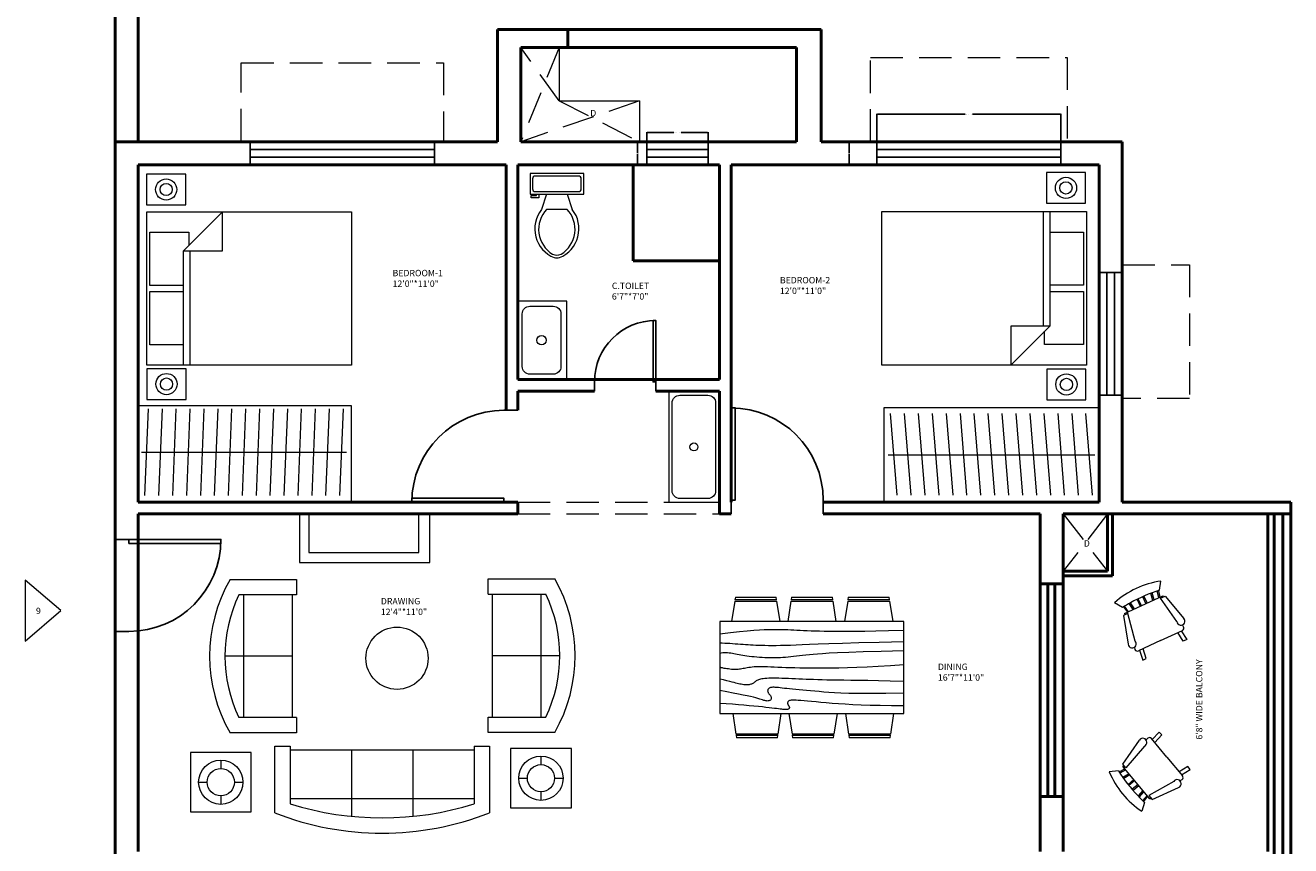
# Model space of a CAD drawing. Units: inches. Extents: x 4795 to 6024, y 2716 to 5025.
# Tile 16 of 19: x 5493 to 5988, y 4094 to 4414. Entities that reach past the tile are written whole.
import ezdxf

# ---------------------------------------------------------------- set-up
doc = ezdxf.new("R2010")
doc.units = ezdxf.units.IN
doc.linetypes.add('DASHED', pattern=[19.05, 12.7, -6.35])
for name, color, linetype, lineweight in [('A-ANNO-DIMS', 2, 'Continuous', 18), ('A-ANNO-TEXT', 7, 'Continuous', 18), ('A-AREA-IDEN', 3, 'Continuous', 18), ('A-DOOR', 4, 'Continuous', 25), ('A-FLOR-FIXT', 9, 'Continuous', 18), ('A-FURN', 8, 'Continuous', 18), ('A-GLAZ', 4, 'Continuous', 25), ('A-WALL', 7, 'Continuous', 50), ('A-WALL-OVHD', 8, 'DASHED', 18)]:
    doc.layers.add(name, color=color, linetype=linetype, lineweight=lineweight)
doc.styles.get("Standard").update_dxf_attribs({"font": 'arial.ttf'})
doc.dimstyles.get("Standard").update_dxf_attribs({"dimtxt": 0.18, "dimasz": 0.18, "dimexe": 0.18, "dimexo": 0.0625, "dimgap": 0.09, "dimtad": 0, "dimtih": 1, "dimtoh": 1, "dimdec": 4, "dimzin": 0, "dimdsep": 46, "dimtxsty": 'Standard', "dimcen": 0.09, "dimadec": 0, "dimazin": 0, "dimtfac": 1, "dimtdec": 4, "dimtofl": 0, "dimtmove": 0, "dimatfit": 3, "dimfxl": 1, "dimtolj": 1, "dimtzin": 0, "dimarcsym": 0})

# ---------------------------------------------------------------- blocks, each defined once
blk = doc.blocks.new('*U2')
for p, q in [((0, 0), (0, -6)), ((40, 0), (40, -6))]:
    blk.add_line(p, q)
blk.add_lwpolyline([(0, 0), (0, 40), (1.75, 40), (1.75, 0)], close=True)
blk.add_arc((0, 0), 40, 0, 90)
blk = doc.blocks.new('Bed - Queen')
for p, q in [((0, -80.00003), (0, 0)), ((0, 0), (59.99999, 0)), ((59.99999, 0), (59.99999, -80.00003)), ((7.99999, -1.2), (28.79998, -1.2)), ((7.99999, -14.4), (7.99999, -1.2)), ((28.79998, -1.2), (28.79998, -14.4)), ((31.19999, -1.2), (51.99999, -1.2)), ((31.19999, -14.4), (31.19999, -1.2)), ((51.99999, -1.2), (51.99999, -16.4)), ((0, -14.4), (44.8, -14.4)), ((59.99999, -29.6), (44.8, -14.4)), ((44.8, -14.4), (44.8, -29.6)), ((44.8, -16.8), (0, -16.8)), ((51.99999, -16.4), (46.79936, -16.4)), ((44.8, -29.6), (59.99999, -29.6)), ((59.99999, -80.00003), (0, -80.00003))]:
    blk.add_line(p, q)
blk = doc.blocks.new('Toilet - top')
for p, q in [((9.5, -6), (9.5, -2)), ((-10, -8.5), (-8, -8.5)), ((-10, -9.5), (-10, -8.5)), ((-7, -9.5), (-10, -9.5)), ((-8, -8.5), (-8, -8)), ((-7, -8), (-7, -9.5)), ((-4, -8), (-6, -14)), ((4, -8), (6, -14)), ((4, -14), (-4, -14))]:
    blk.add_line(p, q)
blk.add_lwpolyline([(10.5, -8), (10.5, 0), (-10.5, 0), (-10.5, -8)], close=True)
for points in [[(-9.5, -2), (-9.5, -6)], [(8.5, -1), (-8.5, -1)], [(-8.5, -7), (8.5, -7)]]:
    blk.add_lwpolyline(points)
for centre, radius, start, end in [((-8.62, -1.88), 0.884, 81.8699, 188.1301), ((8.62, -1.88), 0.884, 351.8699, 98.1301), ((-8.62, -6.12), 0.884, 171.8699, 278.1301), ((8.62, -6.12), 0.884, 261.8699, 8.1301), ((3.52, -21.58), 12.17, 141.4691, 247.9714), ((4.2, -21.82), 11.33, 136.3677, 238.9468), ((-3.52, -21.58), 12.17, 292.0284, 38.5307), ((-4.2, -21.82), 11.33, 301.053, 43.6321), ((0, -27.88), 4, 245.7318, 294.2682), ((0, -29), 4, 254.8605, 285.1395)]:
    blk.add_arc(centre, radius, start, end)
blk = doc.blocks.new('Sofa - Roundback 7 ft.')
for p, q in [((-12.00002, -32.4421), (-12.00003, -6.5971)), ((11.99997, -32.4421), (11.99998, -6.5971)), ((-36.000027, -34), (-36.000027, -11.4696)), ((-35.999844, -13.3819), (35.9998, -13.3819)), ((35.99998, -34), (35.99998, -11.4696)), ((-36.000027, -32.4421), (35.99998, -32.4421))]:
    blk.add_line(p, q)
for points in [[(-36.000027, -34), (-42.000027, -34), (-42.000027, -8)], [(41.99998, -8), (41.99998, -34), (35.99998, -34)]]:
    blk.add_lwpolyline(points)
for centre, radius, start, end in [((0, -114.25), 114.25, 68.43141, 111.5686), ((-0.00001, -127.1968), 121.1968, 72.72033, 107.2797)]:
    blk.add_arc(centre, radius, start, end)
blk = doc.blocks.new('Sofa - Roundback Loveseat 5 ft.')
for p, q in [((0, -32.44198), (0, -5.99998)), ((-24, -33.99998), (-24, -11.46958)), ((-23.9998, -13.38178), (23.99986, -13.38178)), ((24.00004, -33.99998), (24.00004, -11.46958)), ((-24, -32.44198), (24.00004, -32.44198))]:
    blk.add_line(p, q)
for points in [[(-24, -33.99998), (-30, -33.99998), (-30, -7.99998)], [(30.00004, -7.99998), (30.00004, -33.99998), (24.00004, -33.99998)]]:
    blk.add_lwpolyline(points)
for centre, radius, start, end in [((0, -60.24998), 60.24998, 60.13715, 119.8628), ((0, -61.38438), 55.38444, 64.32083, 115.6792)]:
    blk.add_arc(centre, radius, start, end)
blk = doc.blocks.new('Chair - Rocking')
for p, q in [((-8, -4.5), (-10, -1.5)), ((-7.5, -4.5), (-7, -7)), ((-6.5, -7), (-7.02225, -4.43)), ((-4.5, -7), (-4.96674, -4.19951)), ((-4, -7), (-4.40532, -4.16272)), ((-1.5, -4.05012), (-1.5, -7)), ((-1, -7), (-1, -4.05012)), ((1, -7), (1, -4.04655)), ((1.5, -4.05012), (1.5, -7)), ((4, -7), (4.40187, -4.18694)), ((4.5, -7), (4.96761, -4.19437)), ((6.5, -7), (7, -4.4057)), ((7.5, -4.5), (7, -7)), ((8, -4.5), (10, -1.5)), ((-9, -7.5), (-12, -18.49999)), ((-7, -7.5), (-9, -7.5)), ((-9, -18.49999), (-7, -7.5)), ((-8.23428, -6.99939), (-8.3093, -7.47958)), ((-8.23041, -7), (8.23915, -7)), ((7, -7.5), (9, -7.5)), ((9, -18.49999), (7, -7.5)), ((8.31071, -7.48854), (8.23449, -7.00073)), ((9, -7.5), (12, -18.49999)), ((-10.36644, -20.64523), (-10.5, -21.49999)), ((-9, -22.49999), (-9.5, -26.49999)), ((0, -22.49999), (-9.5, -22.49999)), ((-8, -26.49999), (-7.5, -22.49999)), ((0, -22.49999), (9.5, -22.49999)), ((8, -26.49999), (7.5, -22.49999)), ((9, -22.49999), (9.5, -26.49999)), ((10.5, -21.49999), (10.3575, -20.58798)), ((-9.5, -26.49999), (-8, -26.49999)), ((9.5, -26.49999), (8, -26.49999))]:
    blk.add_line(p, q)
for centre, radius, start, end in [((0, -34.08333), 34.08333, 72.93847, 107.0615), ((0, -68.25004), 64.25, 93.92211, 97.15267), ((0, -68.25004), 64.25, 82.84733, 93.92211), ((-10.5, -18.99999), 1.58114, 161.5651, 18.43495), ((10.5, -18.99999), 1.58114, 161.5651, 18.43495), ((-9.5, -21.49999), 1, 180, 270), ((9.5, -21.49999), 1, 270, 0)]:
    blk.add_arc(centre, radius, start, end)
blk = doc.blocks.new('WIN-48')
for p, q in [((0, 0), (0, 48)), ((0, 48), (9, 48)), ((3, 0), (3, 48)), ((6, 48), (6, 0)), ((9, 48), (9, 0)), ((9, 0), (0, 0))]:
    blk.add_line(p, q)
blk = doc.blocks.new('WIN-72')
for p, q in [((0, 0), (0, 9)), ((0, 9), (72, 9)), ((0, 6), (72, 6)), ((72, 9), (72, 0)), ((72, 3), (0, 3)), ((72, 0), (0, 0))]:
    blk.add_line(p, q)
blk = doc.blocks.new('WIN-24')
for p, q in [((0, 0), (0, 9)), ((0, 9), (24, 9)), ((0, 6), (24, 6)), ((24, 9), (24, 0)), ((24, 3), (0, 3)), ((24, 0), (0, 0))]:
    blk.add_line(p, q)
blk = doc.blocks.new('CHAIR-DINING')
for p, q in [((8, 17.72), (0, 18.97)), ((8, 17.71), (8, 1.25)), ((9.5, 17.48), (8.5, 17.64)), ((8.5, 1.33), (8.5, 17.64)), ((9.5, 17.48), (9.5, 1.48)), ((0, 0), (8, 1.25)), ((8.5, 1.33), (9.5, 1.48))]:
    blk.add_line(p, q)
blk = doc.blocks.new('LAMP-SIDE')
for p, q in [((11.88, 20.25), (11.88, 16.92)), ((3.23, 11.6), (6.56, 11.6)), ((17.2, 11.6), (20.54, 11.6)), ((11.88, 6.28), (11.88, 2.94))]:
    blk.add_line(p, q)
blk.add_lwpolyline([(23.76, 23.19), (0, 23.19), (0, 0), (23.76, 0)], close=True)
for radius in [8.66, 5.32]:
    blk.add_circle((11.88, 11.6), radius)
blk = doc.blocks.new('*D31')
at = {"layer": 'A-ANNO-DIMS', "color": 0, "lineweight": -2, "transparency": 16777216}
for p, q in [((5826.23, 4368.87), (5826.23, 4379.79)), ((5826.41, 4379.61), (5860.82, 4379.61)), ((5898.05, 4379.61), (5863.63, 4379.61)), ((5898.23, 4368.87), (5898.23, 4379.79))]:
    blk.add_line(p, q, dxfattribs=at)
at = {"layer": 'A-ANNO-DIMS', "color": 0, "lineweight": 100, "transparency": 16777216}
for points in [[(5826.41, 4379.64), (5826.41, 4379.58), (5826.23, 4379.61)], [(5898.05, 4379.64), (5898.05, 4379.58), (5898.23, 4379.61)]]:
    blk.add_solid(points, dxfattribs=at)
at = {"layer": 'DEFPOINTS', "color": 0, "lineweight": 100, "transparency": 16777216}
for p in [(5826.23, 4379.61), (5826.23, 4368.81), (5898.23, 4368.81)]:
    blk.add_point(p, dxfattribs=at)
at = {"layer": 'A-ANNO-DIMS', "color": 0, "transparency": 16777216, "insert": (5862.23, 4379.61), "char_height": 0.18, "attachment_point": 5}
blk.add_mtext('\\A1;WINDOW 6\'-0" 72 TYP.', dxfattribs=at)
blk = doc.blocks.new('*D32')
at = {"layer": 'A-ANNO-DIMS', "color": 0, "lineweight": -2, "transparency": 16777216}
for p, q in [((5826.16, 4368.81), (5815.25, 4368.81)), ((5815.43, 4368.63), (5815.43, 4364.49)), ((5815.43, 4359.99), (5815.43, 4364.12)), ((5826.16, 4359.81), (5815.25, 4359.81))]:
    blk.add_line(p, q, dxfattribs=at)
at = {"layer": 'A-ANNO-DIMS', "color": 0, "lineweight": 100, "transparency": 16777216}
for points in [[(5815.4, 4368.63), (5815.46, 4368.63), (5815.43, 4368.81)], [(5815.4, 4359.99), (5815.46, 4359.99), (5815.43, 4359.81)]]:
    blk.add_solid(points, dxfattribs=at)
at = {"layer": 'DEFPOINTS', "color": 0, "lineweight": 100, "transparency": 16777216}
for p in [(5826.23, 4368.81), (5815.43, 4359.81), (5826.23, 4359.81)]:
    blk.add_point(p, dxfattribs=at)
at = {"layer": 'A-ANNO-DIMS', "color": 0, "transparency": 16777216, "insert": (5815.43, 4364.31), "char_height": 0.18, "attachment_point": 5}
blk.add_mtext('\\A1;9 TYP.', dxfattribs=at)
blk = doc.blocks.new('*D33')
at = {"layer": 'A-ANNO-DIMS', "color": 0, "lineweight": -2, "transparency": 16777216}
for p, q in [((5736.2, 4368.87), (5736.2, 4372.59)), ((5736.38, 4372.41), (5746.8, 4372.41)), ((5760.02, 4372.41), (5749.61, 4372.41)), ((5760.2, 4368.87), (5760.2, 4372.59))]:
    blk.add_line(p, q, dxfattribs=at)
at = {"layer": 'A-ANNO-DIMS', "color": 0, "lineweight": 100, "transparency": 16777216}
for points in [[(5736.38, 4372.44), (5736.38, 4372.38), (5736.2, 4372.41)], [(5760.02, 4372.44), (5760.02, 4372.38), (5760.2, 4372.41)]]:
    blk.add_solid(points, dxfattribs=at)
at = {"layer": 'DEFPOINTS', "color": 0, "lineweight": 100, "transparency": 16777216}
for p in [(5736.2, 4372.41), (5736.2, 4368.81), (5760.2, 4368.81)]:
    blk.add_point(p, dxfattribs=at)
at = {"layer": 'A-ANNO-DIMS', "color": 0, "transparency": 16777216, "insert": (5748.2, 4372.41), "char_height": 0.18, "attachment_point": 5}
blk.add_mtext('\\A1;WINDOW 2\'-0" 24 TYP.', dxfattribs=at)
blk = doc.blocks.new('*D34')
at = {"layer": 'A-ANNO-DIMS', "color": 0, "lineweight": -2, "transparency": 16777216}
for p, q in [((5736.14, 4368.81), (5732.42, 4368.81)), ((5732.6, 4368.63), (5732.6, 4364.49)), ((5732.6, 4359.99), (5732.6, 4364.12)), ((5736.14, 4359.81), (5732.42, 4359.81))]:
    blk.add_line(p, q, dxfattribs=at)
at = {"layer": 'A-ANNO-DIMS', "color": 0, "lineweight": 100, "transparency": 16777216}
for points in [[(5732.57, 4368.63), (5732.63, 4368.63), (5732.6, 4368.81)], [(5732.57, 4359.99), (5732.63, 4359.99), (5732.6, 4359.81)]]:
    blk.add_solid(points, dxfattribs=at)
at = {"layer": 'DEFPOINTS', "color": 0, "lineweight": 100, "transparency": 16777216}
for p in [(5736.2, 4368.81), (5732.6, 4359.81), (5736.2, 4359.81)]:
    blk.add_point(p, dxfattribs=at)
at = {"layer": 'A-ANNO-DIMS', "color": 0, "transparency": 16777216, "insert": (5732.6, 4364.31), "char_height": 0.18, "attachment_point": 5}
blk.add_mtext('\\A1;9 TYP.', dxfattribs=at)

msp = doc.modelspace()

# ---------------------------------------------------------------- linework, layer by layer
at = {"layer": 'A-FLOR-FIXT'}
for points in [[(5685.72, 4275.81), (5705, 4275.81), (5705, 4306.43), (5685.72, 4306.43)], [(5764.72, 4271.31), (5744.79, 4271.31), (5744.79, 4227.81), (5764.72, 4227.81)]]:
    msp.add_lwpolyline(points, close=True, dxfattribs=at)
for points in [[(5690.48, 4304.5), (5699.64, 4304.5, -0.414214), (5702.64, 4301.5), (5702.64, 4280.91, -0.414214), (5699.64, 4277.91), (5690.48, 4277.91, -0.414214), (5687.48, 4280.91), (5687.48, 4301.5, -0.414214)], [(5749.15, 4269.68), (5760.14, 4269.68, -0.414214), (5763.14, 4266.68), (5763.14, 4232.28, -0.414214), (5760.14, 4229.28), (5749.15, 4229.28, -0.414214), (5746.15, 4232.28), (5746.15, 4266.68, -0.414214)]]:
    msp.add_lwpolyline(points, format="xyb", close=True, dxfattribs=at)
for centre, radius in [((5695.06, 4291.21), 1.86), ((5754.65, 4249.48), 1.56)]:
    msp.add_circle(centre, radius, dxfattribs=at)
at = {"layer": 'A-FURN'}
for p, q in [((5701.94, 4405.65), (5701.94, 4384.8)), ((5701.94, 4384.8), (5733.35, 4384.8)), ((5733.35, 4384.8), (5733.35, 4368.81)), ((5537.22, 4265.7), (5620.55, 4265.7)), ((5539.93, 4230.44), (5541.29, 4264.33)), ((5545.37, 4230.44), (5546.73, 4264.33)), ((5550.82, 4230.44), (5552.18, 4264.33)), ((5556.27, 4230.44), (5557.63, 4264.33)), ((5561.72, 4230.44), (5563.08, 4264.33)), ((5567.16, 4230.44), (5568.52, 4264.33)), ((5572.61, 4230.44), (5573.97, 4264.33)), ((5578.06, 4230.44), (5579.42, 4264.33)), ((5583.5, 4230.44), (5584.86, 4264.33)), ((5588.95, 4230.44), (5590.31, 4264.33)), ((5594.4, 4230.44), (5595.76, 4264.33)), ((5599.84, 4230.44), (5601.2, 4264.33)), ((5605.29, 4230.44), (5606.65, 4264.33)), ((5610.74, 4230.44), (5612.1, 4264.33)), ((5616.19, 4230.44), (5617.55, 4264.33)), ((5620.55, 4265.7), (5620.55, 4227.81)), ((5829.12, 4228.04), (5829.12, 4264.89)), ((5829.12, 4264.89), (5913.22, 4264.89)), ((5831.46, 4262.53), (5834.04, 4230.58)), ((5836.92, 4262.53), (5839.5, 4230.58)), ((5842.38, 4262.53), (5844.95, 4230.58)), ((5847.83, 4262.53), (5850.41, 4230.58)), ((5853.29, 4262.53), (5855.87, 4230.58)), ((5858.75, 4262.53), (5861.33, 4230.58)), ((5864.21, 4262.53), (5866.79, 4230.58)), ((5869.67, 4262.53), (5872.25, 4230.58)), ((5875.12, 4262.53), (5877.7, 4230.58)), ((5880.58, 4262.53), (5883.16, 4230.58)), ((5886.04, 4262.53), (5888.62, 4230.58)), ((5891.5, 4262.53), (5894.08, 4230.58)), ((5896.96, 4262.53), (5899.54, 4230.58)), ((5902.42, 4262.53), (5905, 4230.58)), ((5907.87, 4262.53), (5910.45, 4230.58)), ((5538.6, 4247.38), (5618.73, 4247.38)), ((5830.64, 4246.4), (5911.52, 4246.4)), ((5600.43, 4223.31), (5600.43, 4204.3)), ((5604.07, 4223.31), (5604.07, 4208.13)), ((5647.06, 4208.13), (5647.06, 4223.31)), ((5651.35, 4204.3), (5651.35, 4223.31)), ((5604.07, 4208.13), (5647.06, 4208.13)), ((5600.43, 4204.3), (5651.35, 4204.3)), ((5493.12, 4197.42), (5493.12, 4173.5)), ((5507.01, 4185.46), (5493.12, 4197.42)), ((5493.12, 4173.5), (5507.01, 4185.46)), ((5836.73, 4181.19), (5764.73, 4181.19)), ((5764.73, 4181.19), (5764.73, 4145.19)), ((5836.73, 4145.19), (5836.73, 4181.19)), ((5764.73, 4145.19), (5836.73, 4145.19))]:
    msp.add_line(p, q, dxfattribs=at)
for points in [[(5540.58, 4344.12), (5555.86, 4344.12), (5555.86, 4356.16), (5540.58, 4356.16)], [(5892.55, 4344.76), (5907.83, 4344.76), (5907.83, 4356.79), (5892.55, 4356.79)], [(5540.7, 4268.02), (5555.98, 4268.02), (5555.98, 4280.05), (5540.7, 4280.05)], [(5892.73, 4267.88), (5908.01, 4267.88), (5908.01, 4279.92), (5892.73, 4279.92)]]:
    msp.add_lwpolyline(points, close=True, dxfattribs=at)
for points in [[(5836.73, 4177.69), (5830.82, 4177.52), (5825.76, 4177.4), (5821.46, 4177.32), (5817.81, 4177.26), (5814.7, 4177.24), (5812.03, 4177.23), (5809.7, 4177.25), (5807.61, 4177.27), (5805.65, 4177.31), (5803.82, 4177.35), (5802.1, 4177.4), (5800.49, 4177.45), (5798.97, 4177.51), (5797.53, 4177.57), (5796.18, 4177.63), (5794.9, 4177.69), (5793.68, 4177.75), (5792.5, 4177.81), (5791.34, 4177.87), (5790.18, 4177.91), (5789.01, 4177.95), (5787.8, 4177.98), (5786.53, 4177.99), (5785.19, 4177.98), (5783.74, 4177.95), (5782.12, 4177.89), (5780.25, 4177.79), (5778.07, 4177.63), (5775.5, 4177.4), (5772.47, 4177.1), (5768.9, 4176.7), (5764.73, 4176.19)], [(5836.73, 4173.19), (5827.13, 4173), (5819.2, 4172.82), (5812.71, 4172.64), (5807.47, 4172.47), (5803.25, 4172.31), (5799.85, 4172.17), (5797.05, 4172.04), (5794.65, 4171.94), (5792.45, 4171.86), (5790.43, 4171.8), (5788.56, 4171.76), (5786.84, 4171.73), (5785.24, 4171.72), (5783.77, 4171.73), (5782.41, 4171.75), (5781.15, 4171.77), (5779.97, 4171.81), (5778.86, 4171.85), (5777.81, 4171.9), (5776.8, 4171.96), (5775.82, 4172.02), (5774.85, 4172.08), (5773.88, 4172.16), (5772.9, 4172.23), (5771.88, 4172.31), (5770.85, 4172.39), (5769.8, 4172.47), (5768.75, 4172.54), (5767.71, 4172.6), (5766.69, 4172.65), (5765.69, 4172.68), (5764.73, 4172.69)], [(5836.73, 4169.69), (5827.92, 4169.5), (5820.81, 4169.32), (5815.2, 4169.13), (5810.84, 4168.95), (5807.51, 4168.77), (5804.97, 4168.6), (5802.99, 4168.43), (5801.36, 4168.27), (5799.86, 4168.12), (5798.46, 4167.98), (5797.14, 4167.84), (5795.9, 4167.71), (5794.73, 4167.59), (5793.6, 4167.48), (5792.53, 4167.37), (5791.48, 4167.27), (5790.46, 4167.18), (5789.46, 4167.1), (5788.47, 4167.04), (5787.48, 4166.98), (5786.5, 4166.94), (5785.5, 4166.92), (5784.5, 4166.92), (5783.48, 4166.94), (5782.44, 4166.98), (5781.39, 4167.05), (5780.33, 4167.13), (5779.28, 4167.22), (5778.26, 4167.33), (5777.26, 4167.44), (5776.3, 4167.57), (5775.4, 4167.69), (5774.55, 4167.81), (5773.76, 4167.94), (5773.02, 4168.06), (5772.31, 4168.18), (5771.63, 4168.3), (5770.97, 4168.42), (5770.33, 4168.54), (5769.69, 4168.65), (5769.05, 4168.75), (5768.4, 4168.85), (5767.77, 4168.92), (5767.13, 4168.97), (5766.51, 4168.97), (5765.9, 4168.94), (5765.3, 4168.84), (5764.73, 4168.69)], [(5836.73, 4164.19), (5831.52, 4163.85), (5826.75, 4163.57), (5822.38, 4163.35), (5818.39, 4163.18), (5814.73, 4163.06), (5811.38, 4162.98), (5808.31, 4162.92), (5805.48, 4162.9), (5802.86, 4162.89), (5800.44, 4162.9), (5798.2, 4162.93), (5796.12, 4162.97), (5794.18, 4163.01), (5792.37, 4163.07), (5790.67, 4163.13), (5789.06, 4163.19), (5787.54, 4163.25), (5786.1, 4163.31), (5784.73, 4163.36), (5783.45, 4163.41), (5782.25, 4163.44), (5781.13, 4163.46), (5780.1, 4163.46), (5779.15, 4163.44), (5778.28, 4163.4), (5777.5, 4163.34), (5776.78, 4163.26), (5776.12, 4163.17), (5775.51, 4163.07), (5774.94, 4162.97), (5774.41, 4162.87), (5773.9, 4162.77), (5773.4, 4162.68), (5772.92, 4162.6), (5772.44, 4162.54), (5771.96, 4162.48), (5771.47, 4162.44), (5770.97, 4162.42), (5770.45, 4162.42), (5769.9, 4162.44), (5769.32, 4162.48), (5768.73, 4162.54), (5768.14, 4162.62), (5767.57, 4162.7), (5767.03, 4162.79), (5766.54, 4162.87), (5766.12, 4162.95), (5765.77, 4163.02), (5765.52, 4163.08), (5765.35, 4163.12), (5765.23, 4163.15), (5765.14, 4163.17), (5765.07, 4163.18), (5764.99, 4163.19), (5764.89, 4163.19), (5764.73, 4163.19)], [(5836.73, 4157.69), (5831.45, 4157.86), (5826.8, 4157.98), (5822.73, 4158.07), (5819.16, 4158.14), (5816.03, 4158.18), (5813.28, 4158.22), (5810.84, 4158.24), (5808.65, 4158.27), (5806.64, 4158.31), (5804.79, 4158.35), (5803.07, 4158.4), (5801.47, 4158.45), (5799.96, 4158.51), (5798.51, 4158.57), (5797.11, 4158.63), (5795.73, 4158.69), (5794.36, 4158.75), (5793, 4158.81), (5791.66, 4158.87), (5790.36, 4158.92), (5789.1, 4158.96), (5787.9, 4158.99), (5786.78, 4159.02), (5785.73, 4159.02), (5784.78, 4159.02), (5783.91, 4158.99), (5783.13, 4158.95), (5782.43, 4158.9), (5781.8, 4158.83), (5781.24, 4158.74), (5780.75, 4158.64), (5780.31, 4158.52), (5779.93, 4158.39), (5779.6, 4158.25), (5779.31, 4158.09), (5779.04, 4157.93), (5778.8, 4157.76), (5778.58, 4157.6), (5778.36, 4157.43), (5778.15, 4157.27), (5777.92, 4157.12), (5777.69, 4156.98), (5777.44, 4156.85), (5777.18, 4156.73), (5776.9, 4156.63), (5776.59, 4156.55), (5776.26, 4156.48), (5775.9, 4156.44), (5775.51, 4156.42), (5775.09, 4156.42), (5774.65, 4156.45), (5774.18, 4156.49), (5773.69, 4156.56), (5773.19, 4156.64), (5772.67, 4156.74), (5772.15, 4156.86), (5771.61, 4156.99), (5771.02, 4157.14), (5770.36, 4157.32), (5769.6, 4157.52), (5768.68, 4157.76), (5767.59, 4158.03), (5766.28, 4158.34), (5764.73, 4158.69)], [(5836.73, 4153.19), (5829.71, 4153.05), (5823.9, 4152.99), (5819.16, 4152.99), (5815.3, 4153.05), (5812.17, 4153.16), (5809.61, 4153.3), (5807.45, 4153.45), (5805.52, 4153.61), (5803.7, 4153.76), (5801.96, 4153.9), (5800.29, 4154.04), (5798.7, 4154.18), (5797.2, 4154.31), (5795.79, 4154.44), (5794.46, 4154.56), (5793.23, 4154.69), (5792.09, 4154.81), (5791.04, 4154.94), (5790.08, 4155.05), (5789.2, 4155.16), (5788.4, 4155.25), (5787.69, 4155.33), (5787.05, 4155.4), (5786.48, 4155.44), (5785.98, 4155.46), (5785.55, 4155.46), (5785.18, 4155.43), (5784.86, 4155.39), (5784.58, 4155.32), (5784.35, 4155.24), (5784.15, 4155.14), (5783.98, 4155.02), (5783.84, 4154.89), (5783.72, 4154.74), (5783.62, 4154.59), (5783.55, 4154.42), (5783.51, 4154.24), (5783.5, 4154.06), (5783.52, 4153.88), (5783.56, 4153.69), (5783.64, 4153.5), (5783.74, 4153.31), (5783.87, 4153.13), (5784, 4152.94), (5784.15, 4152.75), (5784.29, 4152.56), (5784.43, 4152.38), (5784.56, 4152.19), (5784.68, 4152), (5784.78, 4151.82), (5784.86, 4151.63), (5784.91, 4151.45), (5784.93, 4151.27), (5784.93, 4151.1), (5784.89, 4150.93), (5784.81, 4150.77), (5784.7, 4150.62), (5784.55, 4150.48), (5784.37, 4150.36), (5784.16, 4150.25), (5783.92, 4150.17), (5783.65, 4150.12), (5783.37, 4150.09), (5783.06, 4150.11), (5782.74, 4150.16), (5782.39, 4150.24), (5781.99, 4150.36), (5781.54, 4150.51), (5781.01, 4150.68), (5780.4, 4150.87), (5779.68, 4151.09), (5778.86, 4151.31), (5777.9, 4151.56), (5776.77, 4151.82), (5775.45, 4152.1), (5773.9, 4152.42), (5772.09, 4152.79), (5769.98, 4153.2), (5767.54, 4153.66), (5764.73, 4154.19)], [(5836.73, 4148.19), (5831.91, 4148.21), (5827.54, 4148.28), (5823.58, 4148.37), (5820.01, 4148.5), (5816.77, 4148.65), (5813.83, 4148.82), (5811.15, 4149), (5808.69, 4149.19), (5806.42, 4149.38), (5804.33, 4149.56), (5802.43, 4149.73), (5800.69, 4149.9), (5799.14, 4150.05), (5797.75, 4150.17), (5796.53, 4150.28), (5795.48, 4150.36), (5794.59, 4150.4), (5793.85, 4150.42), (5793.24, 4150.41), (5792.75, 4150.38), (5792.36, 4150.32), (5792.06, 4150.24), (5791.83, 4150.14), (5791.65, 4150.02), (5791.51, 4149.89), (5791.41, 4149.75), (5791.34, 4149.59), (5791.3, 4149.43), (5791.29, 4149.26), (5791.31, 4149.1), (5791.34, 4148.93), (5791.4, 4148.77), (5791.47, 4148.62), (5791.55, 4148.47), (5791.63, 4148.34), (5791.72, 4148.2), (5791.8, 4148.07), (5791.88, 4147.94), (5791.94, 4147.82), (5791.98, 4147.69), (5792, 4147.57), (5792, 4147.44), (5791.97, 4147.32), (5791.92, 4147.21), (5791.84, 4147.11), (5791.75, 4147.01), (5791.63, 4146.93), (5791.48, 4146.86), (5791.31, 4146.8), (5791.11, 4146.76), (5790.88, 4146.74), (5790.61, 4146.73), (5790.28, 4146.74), (5789.91, 4146.76), (5789.48, 4146.8), (5788.98, 4146.86), (5788.41, 4146.93), (5787.76, 4147.01), (5787.02, 4147.11), (5786.16, 4147.22), (5785.19, 4147.34), (5784.09, 4147.48), (5782.84, 4147.62), (5781.44, 4147.77), (5779.87, 4147.93), (5778.14, 4148.1), (5776.26, 4148.27), (5774.23, 4148.45), (5772.05, 4148.63), (5769.74, 4148.82), (5767.3, 4149), (5764.73, 4149.19)]]:
    msp.add_lwpolyline(points, dxfattribs=at)
for centre, radius in [((5548.22, 4350.14), 4.15), ((5548.22, 4350.14), 2.4), ((5900.19, 4350.78), 4.15), ((5900.19, 4350.78), 2.4), ((5548.34, 4274.04), 4.15), ((5900.37, 4273.9), 4.15), ((5548.34, 4274.04), 2.4), ((5900.37, 4273.9), 2.4), ((5638.52, 4166.82), 12.16)]:
    msp.add_circle(centre, radius, dxfattribs=at)
at = {"layer": 'A-WALL'}
for p, q in [((5528.22, 4507.98), (5528.22, 3920.81)), ((5537.22, 4507.98), (5537.22, 4368.81)), ((5677.84, 4368.81), (5677.84, 4412.75)), ((5677.84, 4412.75), (5804.44, 4412.75)), ((5705.35, 4412.75), (5705.35, 4405.65)), ((5804.44, 4412.75), (5804.44, 4368.81)), ((5686.94, 4368.81), (5686.94, 4405.65)), ((5686.94, 4405.65), (5794.78, 4405.65)), ((5794.78, 4405.65), (5794.78, 4368.81)), ((5528.22, 4368.81), (5677.84, 4368.81)), ((5686.94, 4368.81), (5794.78, 4368.81)), ((5804.44, 4368.81), (5922.22, 4368.81)), ((5922.22, 4368.81), (5922.22, 4227.81)), ((5537.22, 4359.81), (5681.22, 4359.81)), ((5537.22, 4359.81), (5537.22, 4227.81)), ((5681.22, 4359.81), (5681.22, 4263.81)), ((5685.72, 4359.81), (5685.72, 4275.81)), ((5685.72, 4359.81), (5764.72, 4359.81)), ((5730.89, 4359.81), (5730.89, 4322.26)), ((5764.72, 4359.81), (5764.72, 4275.81)), ((5769.22, 4359.81), (5769.22, 4227.81)), ((5769.22, 4359.81), (5913.22, 4359.81)), ((5913.22, 4359.81), (5913.22, 4227.81)), ((5730.89, 4322.26), (5764.72, 4322.26)), ((5685.72, 4275.81), (5764.72, 4275.81)), ((5685.72, 4271.31), (5715.76, 4271.31)), ((5685.72, 4271.31), (5685.72, 4263.81)), ((5739.76, 4271.31), (5764.72, 4271.31)), ((5764.72, 4271.31), (5764.72, 4223.31)), ((5537.22, 4227.81), (5685.72, 4227.81)), ((5685.72, 4227.81), (5685.72, 4223.31)), ((5805.22, 4227.81), (5913.22, 4227.81)), ((5922.22, 4227.81), (5988.09, 4227.81)), ((5988.09, 4227.81), (5988.09, 4086.81)), ((5537.22, 4223.31), (5685.72, 4223.31)), ((5537.22, 4223.31), (5537.22, 4091.31)), ((5764.72, 4223.31), (5769.22, 4223.31)), ((5805.22, 4223.31), (5890.09, 4223.31)), ((5890.09, 4223.31), (5890.09, 4091.31)), ((5899.09, 4223.31), (5899.09, 4091.31)), ((5899.09, 4223.31), (5922.22, 4223.31)), ((5916.47, 4223.31), (5916.47, 4200.83)), ((5918.37, 4223.31), (5918.37, 4199.09)), ((5922.22, 4223.31), (5988.09, 4223.31)), ((5979.09, 4223.31), (5979.09, 4091.31)), ((5981.57, 4223.31), (5981.57, 4090.21)), ((5984.99, 4088.3), (5984.99, 4223.31)), ((5916.47, 4200.83), (5899.09, 4200.83)), ((5918.37, 4199.09), (5899.09, 4199.09)), ((5890.09, 4195.86), (5899.09, 4195.86)), ((5893.11, 4195.86), (5893.11, 4112.75)), ((5895.79, 4195.86), (5895.79, 4112.75)), ((5890.09, 4112.75), (5899.09, 4112.75))]:
    msp.add_line(p, q, dxfattribs=at)
at = {"layer": 'A-WALL-OVHD'}
for p, q in [((5701.94, 4384.8), (5686.94, 4405.65)), ((5701.94, 4405.65), (5686.94, 4368.81)), ((5823.7, 4368.81), (5823.7, 4401.81)), ((5823.7, 4401.81), (5900.65, 4401.81)), ((5900.65, 4401.81), (5900.65, 4368.81)), ((5577.58, 4368.98), (5577.58, 4399.68)), ((5577.58, 4399.68), (5656.65, 4399.68)), ((5656.65, 4399.68), (5656.65, 4368.81)), ((5733.35, 4384.8), (5686.94, 4368.81)), ((5701.94, 4384.8), (5733.35, 4368.81)), ((5922.22, 4320.72), (5948.57, 4320.72)), ((5948.57, 4320.72), (5948.57, 4268.44)), ((5948.57, 4268.44), (5922.22, 4268.44)), ((5685.72, 4227.81), (5764.72, 4227.81)), ((5685.72, 4223.31), (5764.72, 4223.31)), ((5899.09, 4223.31), (5916.47, 4200.83)), ((5916.47, 4223.31), (5899.09, 4200.83))]:
    msp.add_line(p, q, dxfattribs=at)

# ---------------------------------------------------------------- block references
at = {"layer": 'A-DOOR'}
for p, xscale, yscale, zscale in [((5739.76, 4274.91), -0.6, 0.6, 0.6), ((5769.22, 4228.71), 0.9, 0.9, 0.9)]:
    msp.add_blockref('*U2', p, dxfattribs=dict(at, xscale=xscale, yscale=yscale, zscale=zscale))
at = {"layer": 'A-DOOR', "xscale": 0.9, "yscale": 0.9, "zscale": 0.9}
for p, rotation in [((5680.32, 4227.81), 90), ((5533.66, 4213.3), 270)]:
    msp.add_blockref('*U2', p, dxfattribs=dict(at, rotation=rotation))
at = {"layer": 'A-FLOR-FIXT'}
msp.add_blockref('Toilet - top', (5701.04, 4356.36), dxfattribs=at)
at = {"layer": 'A-FURN'}
for name, p, rotation in [('Bed - Queen', (5540.66, 4281.4), 90), ('Bed - Queen', (5908.21, 4341.5), 270), ('Sofa - Roundback Loveseat 5 ft.', (5565.21, 4167.61), 90), ('Sofa - Roundback Loveseat 5 ft.', (5708.21, 4167.84), 270), ('Chair - Rocking', (5927.62, 4194.12), 24.98478846597024), ('CHAIR-DINING', (5788.34, 4181.19), 90.00567182442555), ('CHAIR-DINING', (5810.31, 4181.19), 90.0056718244202), ('CHAIR-DINING', (5832.53, 4181.19), 90.0056718244202), ('CHAIR-DINING', (5769.86, 4145.19), 270.0000000000034), ('CHAIR-DINING', (5791.8, 4145.19), 270.0000000000061), ('CHAIR-DINING', (5813.9, 4145.19), 270.0000000000061), ('Chair - Rocking', (5922.36, 4113.74), 129.6958839725731), ('Sofa - Roundback 7 ft.', (5632.7, 4098.4), 180)]:
    msp.add_blockref(name, p, dxfattribs=dict(at, rotation=rotation))
for p in [(5557.7, 4106.75), (5682.95, 4108.3)]:
    msp.add_blockref('LAMP-SIDE', p, dxfattribs=at)
at = {"layer": 'A-GLAZ', "rotation": 180}
for name, p in [('WIN-72', (5653.14, 4368.81)), ('WIN-24', (5760.2, 4368.81)), ('WIN-72', (5898.23, 4368.81)), ('WIN-48', (5922.22, 4317.65))]:
    msp.add_blockref(name, p, dxfattribs=at)

# ---------------------------------------------------------------- texts
at = {"layer": 'A-ANNO-TEXT', "char_height": 2.5, "attachment_point": 1}
for s, width, insert in [('D', 1.2206, (5714.1, 4381.28)), ('D', 1.6222, (5907.17, 4212.97)), ('9', 4.7591, (5497.3, 4186.6))]:
    msp.add_mtext_dynamic_manual_height_columns(s, width=width, gutter_width=12.5, heights=[0], dxfattribs=dict(at, insert=insert))
at = {"layer": 'A-AREA-IDEN', "char_height": 2.5, "attachment_point": 1}
for s, width, insert in [('BEDROOM-1\\P12\'0"*11\'0"', 48.783, (5636.79, 4318.72)), ('C.TOILET\\P6\'7"*7\'0"', 39.0355, (5722.56, 4313.73)), ('BEDROOM-2\\P12\'0"*11\'0"', 46.1844, (5788.29, 4315.93)), ('DRAWING\\P12\'4"*11\'0"', 39.2679, (5632.2, 4190.39)), ('DINING\\P16\'7"*11\'0"', 39.7145, (5850.11, 4164.73))]:
    msp.add_mtext_dynamic_manual_height_columns(s, width=width, gutter_width=12.5, heights=[0], dxfattribs=dict(at, insert=insert))
at = {"layer": 'A-AREA-IDEN', "insert": (5951.04, 4134.99), "char_height": 2.5, "attachment_point": 1, "rotation": 90}
msp.add_mtext_dynamic_manual_height_columns('6\'8" WIDE BALCONY', width=49.8458, gutter_width=12.5, heights=[0], dxfattribs=at)

# ---------------------------------------------------------------- dimensions: what is measured, and where the dimension line sits
at = {"layer": 'A-ANNO-DIMS'}
for base, p1, p2, angle, text, picture, middle in [((5826.23, 4379.61), (5898.23, 4368.81), (5826.23, 4368.81), 180, 'WINDOW 6\'-0" <> TYP.', '*D31', (5862.23, 4379.61)), ((5736.2, 4372.41), (5760.2, 4368.81), (5736.2, 4368.81), 180, 'WINDOW 2\'-0" <> TYP.', '*D33', (5748.2, 4372.41)), ((5732.6, 4359.81), (5736.2, 4368.81), (5736.2, 4359.81), 270, '<> TYP.', '*D34', (5732.6, 4364.31)), ((5815.43, 4359.81), (5826.23, 4368.81), (5826.23, 4359.81), 270, '<> TYP.', '*D32', (5815.43, 4364.31))]:
    dim = msp.add_linear_dim(base=base, p1=p1, p2=p2, angle=angle, text=text, dimstyle='Standard', override={"dimdec": 0, "dimlfac": 1, "dimrnd": 0, "dimzin": 0, "dimdsep": 46, "dimlunit": 2}, dxfattribs=at)
    dim.commit()
    dim.dimension.update_dxf_attribs({"geometry": picture, "text_midpoint": middle})

doc.saveas('drawing.dxf')
